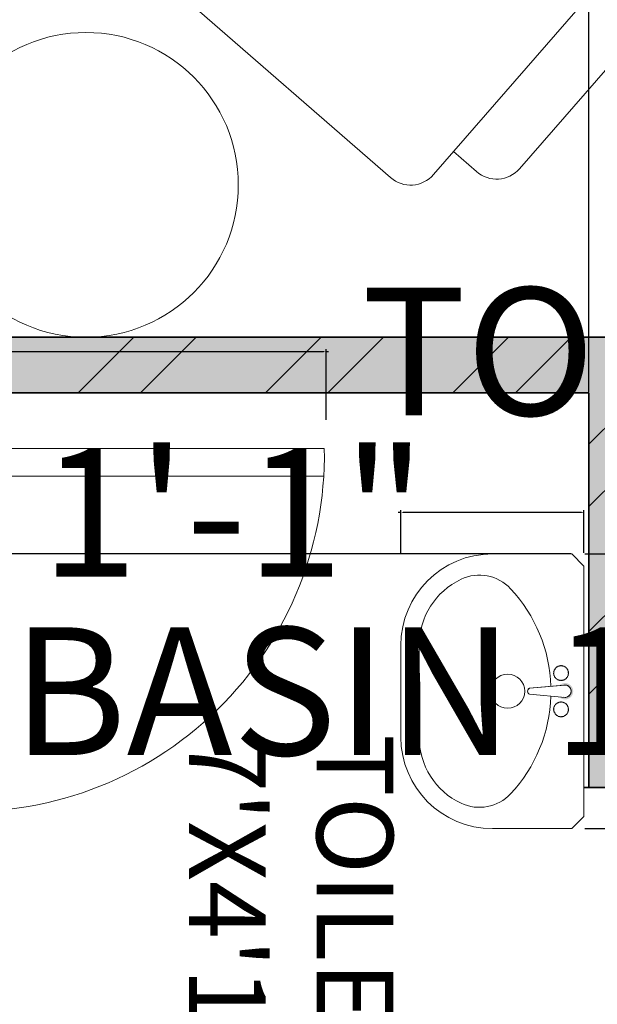
# Model space of a CAD drawing. Units: inches. Extents: x 1086 to 1540, y 3343 to 3848.
# Tile 4 of 8: x 1381 to 1422, y 3591 to 3661. Entities that reach past the tile are written whole.
import ezdxf

# ---------------------------------------------------------------- set-up
doc = ezdxf.new("R2010")
doc.units = ezdxf.units.IN
for name, color, linetype, lineweight in [('00 FURNITURE', 15, 'Continuous', 15), ('A-ANNO-DIMS', 2, 'Continuous', 13), ('A-AREA-IDEN', 7, 'Continuous', 18), ('A-DOOR', 4, 'Continuous', 20), ('A-FLOR-FIXT', 9, 'Continuous', 18), ('A-WALL-PATT', 252, 'Continuous', 9), ('A_FUR 1', 5, 'Continuous', 5), ('WALL', 7, 'Continuous', 35)]:
    doc.layers.add(name, color=color, linetype=linetype, lineweight=lineweight)
doc.styles.get("Standard").update_dxf_attribs({"font": 'arial.ttf'})
doc.dimstyles.get("Standard").update_dxf_attribs({"dimtxt": 9.18, "dimasz": 0.18, "dimexe": 0.18, "dimexo": 0.0625, "dimgap": 0.09, "dimtad": 0, "dimtih": 1, "dimtoh": 1, "dimdec": 1, "dimzin": 0, "dimdsep": 46, "dimlunit": 3, "dimtxsty": 'Standard', "dimcen": 0.09, "dimadec": 0, "dimazin": 0, "dimtfac": 1, "dimtdec": 1, "dimtofl": 0, "dimtmove": 0, "dimatfit": 3, "dimfxl": 1, "dimtolj": 1, "dimtzin": 0, "dimarcsym": 0})

# ---------------------------------------------------------------- blocks, each defined once
blk = doc.blocks.new('s_46')
at = {"ltscale": 600}
h = blk.add_hatch(color=256, dxfattribs=at)
edge = h.paths.add_edge_path()
edge.add_line((13.45184378023259, 62.04360352296498), (14.15927104179718, 54.09782096462731))
edge.add_ellipse((4.212458010588306, 52.31250418393756), major_axis=(-10.10576298371302, 2.5e-15), ratio=1, start_angle=540, end_angle=550.1754626554052, ccw=False)
edge.add_arc((4.212458010588306, 52.31250418393756), 10.10576298371302, 270, 360, ccw=False)
edge.add_line((4.212458010588306, 42.20674120020703), (4.212458010588306, 41.28018079043977))
edge.add_line((4.212458010588306, 41.28018079040339), (11.85106942148559, 41.28018079040339))
edge.add_arc((4.212458010588306, 52.31250418393756), 13.41866400745597, 664.6981342835142, 766.4847699121552)
h.paths.add_polyline_path([(4.212458010588306, 41.28018079040339), (-3.426153400272596, 41.28018079040339, 0.152566653256377), (4.212458010588306, 38.8938401764608)])
h.paths.add_polyline_path([(11.85106942144921, 41.28018079040339), (4.212458010588306, 41.28018079040339), (4.212458010588306, 38.8938401764608, 0.1525666532563772)])
h.paths.add_polyline_path([(-5.734355020395014, 54.09782096461277), (-5.026927758881356, 62.04360352296498, 0.4758332592079194), (-3.426153400272596, 41.28018079040339), (4.212458010588306, 41.28018079040339), (4.212458010588306, 42.20674120020703, -0.4672400657637396)])
for p, q in [((-5.893304973142221, 52.31250418385025), (-0.714987907151226, 110.4750654234667)), ((-5.893304973142221, 52.31250418385025), (-0.714987907151226, 110.4750654234667)), ((9.139903928502463, 110.475065423554), (14.15927104174625, 54.09782096461277)), ((14.31822099431883, 52.31250418385025), (9.139903928502463, 110.475065423554)), ((14.15927104174625, 54.09782096461277), (14.31822099431883, 52.31250418385025))]:
    blk.add_line(p, q, dxfattribs=at)
blk.add_lwpolyline([(-220.7875419894117, 171.2801807903452, -0.4142135623730951), (-70.7875419894117, 321.2801807903452), (79.2124580105883, 321.2801807904325, -0.4142135623730951), (229.2124580105883, 171.2801807904325), (229.2124580105883, 41.28018079040339), (209.2124580107047, 21.2801807904325), (-200.7875419893535, 21.28018079034518), (-220.7875419894117, 41.28018079040339)], format="xyb", close=True, dxfattribs=at)
blk.add_lwpolyline([(12.26164246437838, 75.41187665969483, 0.1816379869150311), (172.1859176590806, 141.5383421540609, 0.3263505073803008), (187.6570333366981, 222.6589125997853, 0.2898144196813102), (79.21245801076293, 291.2801807904325), (-70.78754198923707, 291.2801807903452, 0.2898144196813102), (-179.2321173155214, 222.658912599698, 0.3263505073803008), (-163.7610016377293, 141.5383421540609, 0.1816379869150315), (-3.836726442852523, 75.41187665960751)], format="xyb", dxfattribs=at)
for points in [[(-16.83803374727722, 67.43055756771354), (-17.02338931558188, 67.50428807432763), (-17.22058725368697, 67.56961317334208), (-17.42189012444578, 67.6347039079701), (-17.61956049106084, 67.70773132116301), (-17.80586091603618, 67.79686645595939), (-17.97305396257434, 67.91028035557245), (-18.11578784312587, 68.05326030802098), (-18.23825336818117, 68.21955858168076), (-18.34702699835179, 68.40004368982045), (-18.44868519355077, 68.58558414605795), (-18.54980441438965, 68.76704846357461), (-18.65696112113073, 68.9353051558137), (-18.77673177386168, 69.08122273621848), (-18.91569283319404, 69.19566971814493), (-19.07841429975815, 69.27267628890695), (-19.26144033775199, 69.31891933156292), (-19.45930865121772, 69.34423740339116), (-19.66655694507062, 69.35846906132065), (-19.87772292352747, 69.37145286262967), (-20.08734429115429, 69.39302736415993), (-20.2899587523425, 69.43303112310241), (-20.48010401183274, 69.50130269664805), (-20.65391131333308, 69.60429419830325), (-20.81388605764368, 69.73491196823306), (-20.96412718523061, 69.8826759030926), (-21.10873363655992, 70.03710589953698), (-21.25180435174844, 70.18772185422131), (-21.39743827126222, 70.3240436638007), (-21.54973433539272, 70.43559122501756), (-21.71279148443137, 70.5118844343524), (-21.88955151231494, 70.54600451889564), (-22.07832762773614, 70.54527802669325), (-22.27627589285839, 70.52059283622657), (-22.4805523698451, 70.48283682571491), (-22.68831312085968, 70.44289787355228), (-22.89671420806553, 70.41166385821998), (-23.10291169380071, 70.40002265802468), (-23.30406164005399, 70.41886215136037), (-23.49802141042892, 70.4753938675276), (-23.68545357254334, 70.56212393892929), (-23.86772199510597, 70.66788214896224), (-24.04619054717477, 70.78149828102323), (-24.22222309763311, 70.89180211850908), (-24.39718351518968, 70.98762344472925), (-24.57243566872785, 71.05779204316786), (-24.74934342730558, 71.09113769704709), (-24.92903553397628, 71.08022740500746), (-25.11170022917213, 71.03257702605333), (-25.2972906283685, 70.95943963443278), (-25.48575984616764, 70.8720683044812), (-25.67706099752104, 70.7817161102721), (-25.87114719772944, 70.69963612605352), (-26.0679715613951, 70.63708142607356), (-26.26748720381875, 70.60530508466763), (-26.46941223740578, 70.61182491958607), (-26.67252476507565, 70.64921772302478), (-26.87536788737634, 70.70632503094384), (-27.07648470485583, 70.77198837930337), (-27.27441831788747, 70.8350493038015), (-27.46771182701923, 70.88434934031102), (-27.6549083327991, 70.90873002487933), (-27.83455093560042, 70.8970328932919), (-28.00620139669627, 70.84190539614065), (-28.17349611973623, 70.75121864315588), (-28.34109016874572, 70.63664965887438), (-28.51363860827405, 70.50987546765828), (-28.69579650234664, 70.38257309404435), (-28.89221891516354, 70.26641956248204), (-29.10756091127405, 70.17309189750813), (-29.3464775547036, 70.11426712348475), (-29.61160253512208, 70.0940409177856), (-29.89748404390411, 70.0861835690448), (-30.19664889771957, 70.05688401864609), (-30.50162391323829, 69.9723312081478), (-30.80493590747938, 69.79871407902101), (-31.09911169676343, 69.50222157256212), (-31.37667809793493, 69.0490426304168), (-31.63016192783834, 68.40536619405611), (-32.32050594605971, 68.4500712644367), (-32.84873653826071, 68.3918758847285), (-33.24226493795868, 68.25193804170704), (-33.52850237919483, 68.0514157223224), (-33.73486009566113, 67.8114669136994), (-33.88874932087492, 67.5532496026135), (-34.01758128887741, 67.29792177610216), (-34.14876723336056, 67.06664142102818), (-34.30371923936764, 66.87550954936887), (-34.47985279804561, 66.72039927294827), (-34.66858425136889, 66.59212672835565), (-34.86132994201034, 66.48150805244222), (-35.04950621211901, 66.37935938188457), (-35.22452940384392, 66.27649685335928), (-35.37781585985795, 66.16373660371755), (-35.50078192248475, 66.03189476963598), (-35.58785390376579, 65.87432967920904), (-35.64549799636007, 65.69456842611542), (-35.68319036299363, 65.49868029527715), (-35.7104071660433, 65.2927345718781), (-35.73662456823513, 65.08280054092756), (-35.77131873212056, 64.87494748734753), (-35.82396582007641, 64.67524469623459), (-35.90404199482873, 64.48976145259803), (-36.01774371694773, 64.3227640100813), (-36.15814863995183, 64.17130649695173), (-36.31505471485434, 64.0306400101108), (-36.47825989319244, 63.89601564637269), (-36.63756212632871, 63.76268450255157), (-36.78275936545106, 63.62589767554891), (-36.90364956192207, 63.48090626226621), (-36.99003066710429, 63.32296135951764), (-37.03518227743916, 63.14869254492805), (-37.04631056915969, 62.96024331927765), (-37.03410336375237, 62.7611356638954), (-37.00924848217983, 62.55489156045951), (-36.98243374592858, 62.34503299021162), (-36.96434697631048, 62.13508193491725), (-36.96567599463743, 61.92856037581805), (-36.99710862222128, 61.72899029450491), (-37.06570762058254, 61.53896291530691), (-37.16403551277472, 61.35734643402975), (-37.28102976223454, 61.18207828939194), (-37.40562783187488, 61.0110959201993), (-37.52676718513249, 60.84233676508302), (-37.63338528544409, 60.67373826284892), (-37.7144195958972, 60.50323785204091), (-37.75880757992855, 60.32877297155209), (-37.75920177751686, 60.14875038337777), (-37.72311503690435, 59.96345414296957), (-37.66177528270055, 59.77363762940512), (-37.58641044021351, 59.58005422132555), (-37.5082484340528, 59.38345729780849), (-37.43851718935184, 59.18460023758234), (-37.38844463089481, 58.98423641963745), (-37.36925868364051, 58.78311922278953), (-37.38844463089481, 58.58200202594161), (-37.43851718935184, 58.38163820799673), (-37.5082484340528, 58.18278114777058), (-37.58641044021351, 57.98618422425352), (-37.66177528287517, 57.79260081626126), (-37.72311503690435, 57.6027843026095), (-37.75920177751686, 57.4174880622013), (-37.75880757992855, 57.23746547402697), (-37.7144195958972, 57.06300059353816), (-37.63338528544409, 56.89250018273014), (-37.52676718530711, 56.72390168049606), (-37.40562783187488, 56.55514252537978), (-37.28102976223454, 56.38416015618713), (-37.16403551277472, 56.20889201154932), (-37.06570762058254, 56.02727553035947), (-36.99710862222128, 55.83724815107416), (-36.96567599463743, 55.63767806976102), (-36.96434697631048, 55.43115651066182), (-36.98243374592858, 55.22120545536745), (-37.00924848217983, 55.01134688520687), (-37.03410336375237, 54.80510278168367), (-37.04631056933431, 54.60599512638873), (-37.03518227743916, 54.41754590065102), (-36.99003066710429, 54.24327708606142), (-36.90364956192207, 54.08533218331285), (-36.78275936545106, 53.94034077003016), (-36.63756212632871, 53.80355394302751), (-36.47825989319244, 53.67022279920639), (-36.31505471502896, 53.53559843546827), (-36.15814863995183, 53.39493194862734), (-36.01774371712236, 53.24347443549777), (-35.90404199482873, 53.07647699298104), (-35.82396582007641, 52.89099374934449), (-35.77131873212056, 52.69129095823155), (-35.73662456823513, 52.48343790465151), (-35.71040716621792, 52.27350387370098), (-35.68319036299363, 52.06755815021461), (-35.64549799653469, 51.87167001946363), (-35.58785390376579, 51.69190876637003), (-35.50078192248475, 51.53434367594309), (-35.3778353385278, 51.40284301002975), (-35.22468523163116, 51.29247093791491), (-35.05003213009331, 51.19609060572111), (-34.86257656256203, 51.10656515930895), (-34.67101905716118, 51.01675774488831), (-34.48406014236389, 50.91953150840708), (-34.31040034646867, 50.80774959607516), (-34.15874019777402, 50.67427515375311), (-34.03505195630714, 50.51453334218241), (-33.93439480883535, 50.3341973797942), (-33.84909967368003, 50.14150249981321), (-33.77149746881332, 49.94468393520219), (-33.69391911290586, 49.75197691909852), (-33.60869552427903, 49.57161668455228), (-33.50815762107959, 49.41183846470085), (-33.38463632145431, 49.28087749250699), (-33.23284944484476, 49.18408373402781), (-33.05706241185544, 49.11526608630083), (-32.86392754490953, 49.06534817945794), (-32.66009716555709, 49.02525364354369), (-32.45222359569743, 48.98590610860265), (-32.24695915722987, 48.93822920459206), (-32.05095617187908, 48.87314656155649), (-31.870866961719, 48.78158180962782), (-31.71133844077122, 48.65761859554914), (-31.5689958925941, 48.50798063381808), (-31.43845919286832, 48.34255165536887), (-31.31434821744915, 48.17121539139771), (-31.19128284219187, 48.00385557310073), (-31.06388294277713, 47.85035593167413), (-30.92676839523483, 47.72060019822674), (-30.77455907507101, 47.62447210386745), (-30.60346923320321, 47.56846716045401), (-30.41609062027419, 47.54552800310193), (-30.21660936163971, 47.54520904741366), (-30.00921158283018, 47.55706470907898), (-29.79808340937598, 47.570649403875), (-29.58741096680751, 47.57551754757878), (-29.38138038065517, 47.56122355579281), (-29.18417777627474, 47.51732184420689), (-28.99883273948217, 47.43692629240103), (-28.8237486963626, 47.32738863455597), (-28.65617253311211, 47.19962006882997), (-28.49335113610141, 47.06453179311938), (-28.33253139152657, 46.9330350055825), (-28.1709601857583, 46.81604090429027), (-28.00588440499268, 46.72446068713907), (-27.83455093577504, 46.66920555219985), (-27.6549083327991, 46.65750842061243), (-27.46771182701923, 46.68188910518074), (-27.27441831788747, 46.73118914177758), (-27.07648470485583, 46.7942500662757), (-26.87536788755096, 46.85991341454792), (-26.67252476525027, 46.91702072246698), (-26.4694122375804, 46.95441352590569), (-26.26748720399337, 46.96093336082412), (-26.06797156156972, 46.9291570194182), (-25.87114719772944, 46.86660231943824), (-25.67706099769566, 46.78452233530697), (-25.48575984616764, 46.69417014101054), (-25.2972906283685, 46.60679881105898), (-25.11170022934675, 46.53366141943843), (-24.92903553397628, 46.4860110404843), (-24.74934342730558, 46.47510074844467), (-24.57243566890247, 46.50844640232389), (-24.39718351536431, 46.57861500076251), (-24.22222309780773, 46.67443632698268), (-24.0461905473494, 46.78474016446853), (-23.86772199528059, 46.89835629652953), (-23.68545357254334, 47.00411450656247), (-23.49802141060354, 47.09084457796416), (-23.30406164022861, 47.14737629413138), (-23.10291169380071, 47.16621578746708), (-22.89671420806553, 47.15457458727178), (-22.68831312085968, 47.12334057193948), (-22.4805523698451, 47.08340161977685), (-22.27627589285839, 47.04564560926519), (-22.07832762791077, 47.02096041871118), (-21.88955151248956, 47.02023392650881), (-21.71279148443137, 47.05435401113937), (-21.54973433539272, 47.1306472204742), (-21.39743827126222, 47.24219478160375), (-21.25180435174844, 47.37851659118314), (-21.10873363655992, 47.52913254586746), (-20.96412718540523, 47.68356254231185), (-20.81388605764368, 47.83132647717138), (-20.65391131333308, 47.9619442471012), (-20.48010401200736, 48.0649357488437), (-20.28995875251712, 48.13320732230204), (-20.08734429115429, 48.17321108133183), (-19.87772292352747, 48.1947855828621), (-19.66655694507062, 48.2077693840838), (-19.45930865139235, 48.2220010421006), (-19.26144033775199, 48.24731911384152), (-19.07841429993277, 48.29356215667212), (-18.91569283319404, 48.37056872743414), (-18.77673177403631, 48.48501570936059), (-18.65696112113073, 48.63093328976538), (-18.54980441456428, 48.79918998200446), (-18.44868519372539, 48.98065429960843), (-18.34702699835179, 49.16619475575862), (-18.2382533683558, 49.34667986398562), (-18.11578784312587, 49.5129781376454), (-17.97305396274896, 49.6559580900066), (-17.8058609162108, 49.76937198961969), (-17.61956049106084, 49.85850712450337), (-17.4218901246204, 49.93153453769628), (-17.22058725368697, 49.996625272237), (-17.02338931558188, 50.06195037133875), (-16.83803374727722, 50.13568087795284), (-16.67225798609434, 50.22598783511785), (-16.53379946883069, 50.34104228604701), (-16.42766593385022, 50.48645191569812), (-16.34794632298872, 50.65757097714231), (-16.28599987912457, 50.84719036528259), (-16.23318584513618, 51.04810097528389), (-16.18086346407654, 51.25309370196191), (-16.12039197882404, 51.45495944039431), (-16.04313063243171, 51.64648908557137), (-15.94043866742868, 51.82047353248345), (-15.8067031877581, 51.97190354572376), (-15.64842273970134, 52.10456936812261), (-15.47512373042991, 52.22446111202589), (-15.29633256676607, 52.33756888969219), (-15.12157565605594, 52.44988281364204), (-14.96037940529641, 52.567392996134), (-14.82227022130973, 52.69608954960131), (-14.71677451161667, 52.84196258638985), (-14.6501372611965, 53.00919824198354), (-14.61547776852967, 53.19476674450561), (-14.60263391025364, 53.3938343450427), (-14.60144356318051, 53.60156729485606), (-14.60174460412236, 53.81313184503233), (-14.59337490954203, 54.02369424700736), (-14.566172356077, 54.22842075169319), (-14.50997482053935, 54.42247761052567), (-14.41809999983525, 54.6024088327249), (-14.29778487142175, 54.77026946117985), (-14.1597462335485, 54.92949229647638), (-14.01470088359201, 55.08351013963693), (-13.87336561962729, 55.23575579150929), (-13.7464572393801, 55.38966205302859), (-13.64469254092546, 55.54866172495531), (-13.5787883218145, 55.71618760822457), (-13.55583441938506, 55.89474125843844), (-13.56841282837558, 56.08309925056528), (-13.60547858278733, 56.27910691397847), (-13.65598671662155, 56.48060957840062), (-13.70889226370491, 56.68545257346704), (-13.7531502583879, 56.89148122872575), (-13.7777157346718, 57.09654087381204), (-13.77154372638324, 57.29847683827393), (-13.72730239736847, 57.49560352915432), (-13.65251243085367, 57.68811166286468), (-13.55840763938613, 57.8766610333987), (-13.45622183586238, 58.06191143448813), (-13.35718883317895, 58.24452266012667), (-13.27254244388314, 58.42515450413339), (-13.2135164810461, 58.60446676041465), (-13.19134475721512, 58.78311922278953), (-13.2135164810461, 58.96177168516442), (-13.27254244388314, 59.14108394144569), (-13.35718883317895, 59.3217157854524), (-13.45622183586238, 59.50432701109093), (-13.55840763938613, 59.68957741218037), (-13.65251243085367, 59.87812678271438), (-13.72730239736847, 60.07063491642475), (-13.77154372638324, 60.26776160730515), (-13.7777157346718, 60.46969757176703), (-13.7531502583879, 60.67475721685332), (-13.70889226370491, 60.88078587211203), (-13.65598671662155, 61.08562886717845), (-13.60547858278733, 61.2871315316006), (-13.56841282837558, 61.48313919501379), (-13.55583441938506, 61.67149718714063), (-13.5787883218145, 61.8500508373545), (-13.64469254092546, 62.01757672062377), (-13.7464572393801, 62.17657639255048), (-13.87336561962729, 62.33048265406978), (-14.01470088359201, 62.48272830594214), (-14.15974623337388, 62.63674614910269), (-14.29778487142175, 62.79596898448653), (-14.41809999983525, 62.96382961285416), (-14.50997482053935, 63.14376083514071), (-14.566172356077, 63.33781769388588), (-14.59337490936741, 63.5425441985717), (-14.60174460412236, 63.75310660054674), (-14.60144356318051, 63.96467115081032), (-14.60263391025364, 64.17240410053635), (-14.61547776835505, 64.37147170116077), (-14.65013726102188, 64.55704020359553), (-14.71677451144205, 64.7242758591892), (-14.82227022130973, 64.87014889597776), (-14.96037940529641, 64.99884544944507), (-15.12157565605594, 65.11635563193704), (-15.29633256676607, 65.22866955588688), (-15.47512373042991, 65.3417773336405), (-15.64842273970134, 65.46166907745646), (-15.8067031877581, 65.59433489985531), (-15.94043866742868, 65.74576491309563), (-16.04313063225709, 65.9197493600077), (-16.12039197882404, 66.11127900527208), (-16.18086346407654, 66.31314474370447), (-16.23318584513618, 66.5181374703825), (-16.28599987912457, 66.71904808029649), (-16.34794632298872, 66.90866746843676), (-16.42766593385022, 67.07978652988095), (-16.53379946883069, 67.22519615953206), (-16.67225798609434, 67.34025061046123)], [(22.08090273779817, 61.08562886709115), (22.03039460413856, 61.2871315315133), (21.99332884972682, 61.48313919501379), (21.9807504407363, 61.67149718705331), (22.00370434316574, 61.85005083726719), (22.06960856210208, 62.01757672053645), (22.17137326073134, 62.17657639246318), (22.29828164080391, 62.33048265398247), (22.43961690476863, 62.48272830585483), (22.58466225472512, 62.63674614901538), (22.72270089277299, 62.79596898439923), (22.84301602118649, 62.96382961276686), (22.93489084189059, 63.1437608350534), (22.99108837742824, 63.33781769379857), (23.01829093071865, 63.5425441985717), (23.0266606254736, 63.75310660045943), (23.02635958453175, 63.96467115072301), (23.02754993160488, 64.17240410053635), (23.04039378970629, 64.37147170107346), (23.07505328237312, 64.55704020350822), (23.14169053279329, 64.72427585910191), (23.24718624266097, 64.87014889589045), (23.38529542664764, 64.99884544935776), (23.54649167740717, 65.11635563193704), (23.7212485881173, 65.22866955579956), (23.90003975178115, 65.34177733355318), (24.07333876105258, 65.46166907736915), (24.23161920910934, 65.594334899768), (24.36535468877992, 65.74576491300832), (24.46804665360833, 65.9197493600077), (24.54530800017528, 66.11127900518477), (24.60577948542777, 66.31314474361714), (24.65810186648742, 66.51813747029519), (24.71091590047581, 66.71904808020918), (24.77286234433996, 66.90866746834945), (24.85258195520146, 67.07978652979364), (24.95871549018193, 67.22519615953206), (25.09717400744558, 67.34025061046123), (25.26294976862846, 67.43055756771354), (25.44830533693312, 67.50428807432763), (25.64550327503821, 67.56961317334208), (25.84680614579702, 67.6347039079701), (26.04447651241208, 67.70773132116301), (26.23077693756204, 67.79686645595939), (26.3979699841002, 67.91028035557245), (26.54070386447711, 68.05326030802098), (26.66316938970704, 68.21955858168076), (26.77194301970303, 68.40004368982045), (26.87360121507663, 68.58558414605795), (26.97472043591552, 68.76704846357461), (27.08187714248197, 68.9353051558137), (27.20164779538754, 69.08122273621848), (27.34060885454528, 69.19566971814493), (27.50333032128401, 69.27267628890695), (27.68635635910323, 69.31891933165025), (27.88422467274358, 69.34423740347847), (28.09147296642186, 69.35846906140794), (28.30263894487871, 69.37145286262967), (28.51226031250553, 69.39302736424725), (28.71487477386836, 69.43303112318972), (28.90502003318398, 69.50130269673537), (29.07882733468432, 69.60429419839056), (29.23880207899492, 69.73491196832038), (29.38904320658185, 69.88267590317992), (29.53364965791116, 70.0371058996243), (29.67672037309967, 70.18772185430862), (29.82235429261346, 70.324043663888), (29.97465035674395, 70.43559122501756), (30.1377075057826, 70.51188443443971), (30.31446753366618, 70.54600451898295), (30.50324364908738, 70.54527802678058), (30.70119191420963, 70.52059283622657), (30.90546839119634, 70.48283682571491), (31.11322914221091, 70.4428978736396), (31.32163022941677, 70.41166385830729), (31.52782771515195, 70.400022658112), (31.72897766157985, 70.41886215144768), (31.92293743178016, 70.4753938675276), (32.11036959389458, 70.56212393892929), (32.29263801663183, 70.66788214896224), (32.47110656870063, 70.78149828102323), (32.64713911898434, 70.89180211850908), (32.82209953654092, 70.98762344481656), (32.99735169025371, 71.05779204316786), (33.17425944865681, 71.09113769704709), (33.35395155532751, 71.08022740500746), (33.53661625069799, 71.03257702605333), (33.72220664971974, 70.9594396345201), (33.91067586751888, 70.8720683044812), (34.1019770190469, 70.7817161102721), (34.29606321908068, 70.69963612605352), (34.49288758292096, 70.63708142616088), (34.69240322534461, 70.60530508466763), (34.89432825893164, 70.61182491958607), (35.09744078660151, 70.64921772302478), (35.3002839089022, 70.70632503103116), (35.50140072620707, 70.77198837930337), (35.6993343392387, 70.8350493038015), (35.89262784837047, 70.88434934039833), (36.07982435415034, 70.90873002487933), (36.25946695695166, 70.8970328932919), (36.43111741804751, 70.84190539614065), (36.59841214108747, 70.75121864315588), (36.76600619009696, 70.63664965887438), (36.93855462962529, 70.50987546765828), (37.12071252369788, 70.38257309404435), (37.3171349366894, 70.26641956248204), (37.53247693262529, 70.17309189750813), (37.77139357605483, 70.11426712348475), (38.03651855647331, 70.0940409177856), (38.32240006525535, 70.0861835690448), (38.62156491907081, 70.05688401864609), (38.92653993476415, 69.9723312081478), (39.22985192883061, 69.79871407893368), (39.52402771811467, 69.50222157256212), (39.80159411928616, 69.0490426304168), (40.05507794918957, 68.4053661939688), (40.74542196741094, 68.4500712644367), (41.27365255961194, 68.3918758846412), (41.66718095948453, 68.25193804161972), (41.95341840054607, 68.0514157223224), (42.15977611701236, 67.8114669136121), (42.31366534240078, 67.5532496025262), (42.44249731022864, 67.29792177601485), (42.57368325471179, 67.06664142094087), (42.72863526071887, 66.87550954936887), (42.90476881939684, 66.72039927286096), (43.09350027272012, 66.59212672826834), (43.28624596336157, 66.48150805235491), (43.47442223347025, 66.37935938179726), (43.64944542536977, 66.27649685335928), (43.80273188138381, 66.16373660371755), (43.92569794383598, 66.03189476963598), (44.01276992511703, 65.87432967912173), (44.0704140177113, 65.69456842602813), (44.10810638434486, 65.49868029527715), (44.13532318739453, 65.2927345718781), (44.16154058958636, 65.08280054084025), (44.19623475347179, 64.87494748726021), (44.24888184142765, 64.67524469614727), (44.32895801617997, 64.48976145251072), (44.44265973829897, 64.32276400999397), (44.58306466130307, 64.17130649695173), (44.73997073620558, 64.03064001002348), (44.90317591454368, 63.89601564628538), (45.06247814767994, 63.76268450246425), (45.20767538680229, 63.6258976754616), (45.3285655832733, 63.4809062621789), (45.41494668845553, 63.32296135943034), (45.46009829879039, 63.14869254484074), (45.47122659051092, 62.96024331919034), (45.45901938492898, 62.76113566380809), (45.43416450353106, 62.5548915603722), (45.40734976727981, 62.34503299021162), (45.38926299766171, 62.13508193482994), (45.39059201598866, 61.92856037573074), (45.42202464357251, 61.7289902944176), (45.49062364193377, 61.53896291521959), (45.58895153412595, 61.35734643394243), (45.70594578341115, 61.18207828939194), (45.83054385322611, 61.01109592011198), (45.95168320648371, 60.84233676508302), (46.05830130679533, 60.67373826276162), (46.13933561724843, 60.50323785204091), (46.18372360127978, 60.32877297146479), (46.1841177988681, 60.14875038329046), (46.14803105825558, 59.96345414296957), (46.08669130405178, 59.77363762931782), (46.01132646156474, 59.58005422123824), (45.93316445540404, 59.38345729772118), (45.86343321070308, 59.18460023749503), (45.81336065224604, 58.98423641955014), (45.79417470499175, 58.78311922270222), (45.81336065224604, 58.58200202585431), (45.86343321070308, 58.38163820790942), (45.93316445540404, 58.18278114777058), (46.01132646156474, 57.98618422416621), (46.08669130405178, 57.79260081617394), (46.14803105808095, 57.6027843025222), (46.1841177988681, 57.4174880622013), (46.18372360127978, 57.23746547393966), (46.13933561724843, 57.06300059345085), (46.05830130679533, 56.89250018273014), (45.95168320648371, 56.72390168040874), (45.83054385322611, 56.55514252529247), (45.70594578341115, 56.38416015609982), (45.58895153412595, 56.20889201154932), (45.49062364193377, 56.02727553027216), (45.42202464339789, 55.83724815107416), (45.39059201598866, 55.63767806976102), (45.38926299766171, 55.43115651066182), (45.40734976727981, 55.22120545528014), (45.43416450335644, 55.01134688511957), (45.45901938492898, 54.80510278159636), (45.47122659051092, 54.60599512630142), (45.46009829879039, 54.41754590056371), (45.41494668845553, 54.24327708597411), (45.32856558309868, 54.08533218322554), (45.20767538662767, 53.94034076994285), (45.06247814750532, 53.8035539429402), (44.90317591454368, 53.67022279920639), (44.73997073620558, 53.53559843538096), (44.58306466130307, 53.39493194854004), (44.44265973829897, 53.24347443541046), (44.32895801617997, 53.07647699298104), (44.24888184125302, 52.89099374934449), (44.19623475329717, 52.69129095823155), (44.16154058958636, 52.48343790465151), (44.13532318739453, 52.27350387361366), (44.10810638434486, 52.06755815021461), (44.0704140177113, 51.87167001946363), (44.01276992511703, 51.69190876628272), (43.92569794366136, 51.53434367585578), (43.80275135970442, 51.40284301002975), (43.64960125280776, 51.29247093791491), (43.47494815144455, 51.1960906056338), (43.28749258373863, 51.10656515922165), (43.09593507851241, 51.01675774480099), (42.90897616371512, 50.91953150840708), (42.73531636764528, 50.80774959598784), (42.58365621895063, 50.67427515375311), (42.45996797765838, 50.51453334218241), (42.35931083018658, 50.3341973797942), (42.27401569485664, 50.14150249981321), (42.19641349016455, 49.94468393520219), (42.1188351342571, 49.75197691909852), (42.03361154545564, 49.57161668455228), (41.9330736422562, 49.41183846461354), (41.80955234280554, 49.28087749250699), (41.65776546602137, 49.1840837339405), (41.48197843320668, 49.11526608630083), (41.28884356608614, 49.06534817945794), (41.0850131867337, 49.02525364354369), (40.87713961687405, 48.98590610851534), (40.67187517840648, 48.93822920459206), (40.47587219323031, 48.87314656155649), (40.29578298289561, 48.78158180962782), (40.13625446194782, 48.65761859554914), (39.99391191377072, 48.50798063373076), (39.86337521404493, 48.34255165528157), (39.73926423862577, 48.17121539139771), (39.61619886336848, 48.00385557310073), (39.48879896395374, 47.85035593167413), (39.35168441641144, 47.72060019813944), (39.19947509624762, 47.62447210378013), (39.02838525455445, 47.56846716045401), (38.8410066414508, 47.54552800310193), (38.64152538281633, 47.54520904732635), (38.43412760400679, 47.55706470907898), (38.22299943072721, 47.570649403875), (38.01232698798413, 47.57551754757878), (37.80629640183179, 47.56122355579281), (37.60909379745135, 47.51732184420689), (37.42374876065878, 47.43692629240103), (37.24866471753922, 47.32738863455597), (37.08108855428873, 47.19962006882997), (36.91826715727803, 47.06453179311938), (36.75744741270319, 46.9330350056698), (36.59587620693492, 46.81604090429027), (36.4308004261693, 46.72446068713907), (36.25946695695166, 46.66920555228716), (36.07982435397571, 46.65750842061243), (35.89262784837047, 46.68188910518074), (35.6993343392387, 46.73118914177758), (35.50140072620707, 46.7942500662757), (35.30028390872758, 46.85991341454792), (35.09744078642689, 46.91702072246698), (34.89432825875701, 46.954413525993), (34.69240322516998, 46.96093336082412), (34.49288758274633, 46.9291570194182), (34.29606321908068, 46.86660231943824), (34.10197701887228, 46.78452233530697), (33.91067586734425, 46.69417014109785), (33.72220664971974, 46.60679881105898), (33.53661625052337, 46.53366141943843), (33.35395155515289, 46.4860110404843), (33.17425944865681, 46.47510074844467), (32.99735169007909, 46.5084464024112), (32.82209953654092, 46.57861500076251), (32.64713911898434, 46.67443632707), (32.47110656852601, 46.78474016446853), (32.2926380164572, 46.89835629661684), (32.11036959389458, 47.00411450664979), (31.92293743178016, 47.09084457805147), (31.72897766140522, 47.14737629413138), (31.52782771497732, 47.16621578746708), (31.32163022941677, 47.15457458727178), (31.11322914203629, 47.12334057193948), (30.90546839102171, 47.08340161986416), (30.70119191420963, 47.0456456093525), (30.50324364908738, 47.02096041879849), (30.31446753366618, 47.02023392659611), (30.1377075057826, 47.05435401113937), (29.97465035674395, 47.13064722056151), (29.82235429261346, 47.24219478169106), (29.67672037309967, 47.37851659127045), (29.53364965791116, 47.52913254595478), (29.38904320658185, 47.68356254239916), (29.2388020788203, 47.8313264772587), (29.0788273345097, 47.96194424718851), (28.90502003318398, 48.06493574893102), (28.71487477369374, 48.13320732238935), (28.51226031250553, 48.17321108133183), (28.30263894487871, 48.19478558294941), (28.09147296642186, 48.20776938417111), (27.88422467256896, 48.22200104218791), (27.68635635892861, 48.24731911392882), (27.50333032110939, 48.29356215667212), (27.34060885454528, 48.37056872743414), (27.20164779521292, 48.48501570936059), (27.08187714248197, 48.63093328976538), (26.97472043574089, 48.79918998200446), (26.87360121490201, 48.98065429960843), (26.77194301952841, 49.16619475575862), (26.66316938953241, 49.34667986398562), (26.54070386447711, 49.51297813755809), (26.39796998392558, 49.6559580900066), (26.23077693738742, 49.76937198961969), (26.04447651223745, 49.85850712450337), (25.84680614579702, 49.93153453769628), (25.64550327486359, 49.996625272237), (25.44830533675849, 50.06195037133875), (25.26294976862846, 50.13568087795284), (25.09717400727095, 50.22598783520516), (24.95871549018193, 50.34104228604701), (24.85258195520146, 50.48645191561082), (24.77286234416534, 50.657570977055), (24.71091590030119, 50.84719036519527), (24.65810186648742, 51.04810097519657), (24.60577948542777, 51.2530937018746), (24.54530800017528, 51.45495944030699), (24.46804665360833, 51.64648908548406), (24.36535468877992, 51.82047353239614), (24.23161920910934, 51.97190354572376), (24.07333876105258, 52.1045693680353), (23.90003975160653, 52.22446111193858), (23.7212485881173, 52.33756888960488), (23.54649167740717, 52.44988281355472), (23.38529542647302, 52.56739299604669), (23.24718624266097, 52.696089549514), (23.14169053279329, 52.84196258630254), (23.07505328237312, 53.00919824189623), (23.04039378970629, 53.1947667444183), (23.02754993160488, 53.39383434495539), (23.02635958453175, 53.60156729476876), (23.02666062529898, 53.81313184503233), (23.01829093071865, 54.02369424692006), (22.99108837725362, 54.22842075169319), (22.93489084171597, 54.42247761043836), (22.84301602101186, 54.6024088327249), (22.72270089277299, 54.77026946109254), (22.58466225472512, 54.92949229638907), (22.43961690476863, 55.08351013963693), (22.29828164080391, 55.23575579150929), (22.17137326073134, 55.38966205294127), (22.06960856210208, 55.548661724868), (22.00370434316574, 55.71618760813726), (21.9807504407363, 55.89474125843844), (21.99332884972682, 56.08309925047797), (22.03039460413856, 56.27910691389115), (22.08090273779817, 56.48060957840062), (22.13380828505615, 56.68545257346704), (22.17806627973914, 56.89148122872575), (22.20263175602304, 57.09654087381204), (22.19645974773448, 57.29847683827393), (22.15221841871971, 57.49560352915432), (22.07742845220491, 57.68811166286468), (21.98332366073737, 57.87666103331139), (21.88113785721362, 58.06191143448813), (21.78210485453019, 58.24452266012667), (21.69745846523438, 58.42515450413339), (21.63843250239734, 58.60446676032734), (21.61626077856636, 58.78311922270222), (21.63843250239734, 58.96177168507711), (21.69745846523438, 59.14108394135837), (21.78210485453019, 59.32171578536508), (21.88113785721362, 59.50432701100362), (21.98332366073737, 59.68957741209306), (22.07742845220491, 59.87812678262708), (22.15221841871971, 60.07063491633743), (22.19645974773448, 60.26776160721784), (22.20263175602304, 60.46969757167971), (22.17806627973914, 60.67475721676601), (22.13380828505615, 60.88078587202471)]]:
    blk.add_lwpolyline(points, close=True, dxfattribs=at)
blk.add_circle((4.212458010588306, 146.2801807904034), 28, dxfattribs=at)
for centre, radius, start, end in [((4.212458010588306, 108.2109541267855), 5.422722861947412, 24.67830004152974, 155.3216999584702), ((4.212458010588306, 52.31250418393756), 10.10576298371233, 169.8245373479931, 0)]:
    blk.add_arc(centre, radius, start, end, dxfattribs=at)
for centre, major_axis, ratio, start_param, end_param in [((4.212458010762929, 110.475065423554), (-4.927445917859709, 1.2e-15), 0.6410240960233505, 3.141592653589793, 6.283185307179586), ((4.212458010588306, 52.31250418393756), (-10.10576298371302, 2.5e-15), 1, 6.105589980929039, 9.602373287019926)]:
    blk.add_ellipse(centre, major_axis=major_axis, ratio=ratio, start_param=start_param, end_param=end_param, dxfattribs=at)
blk = doc.blocks.new('ESTSET')
at = {"layer": 'A_FUR 1'}
for p, q in [((-10.44359699611232, 4.096573562603225), (-10.44359699611232, 32.09657356260323)), ((-8.44359699611232, 4.096573562603225), (-8.44359699611232, 32.09657356260323)), ((-36.44359699611232, 6.096573562603225), (-36.44359699611232, 3.096573562603225)), ((-34.44359699611232, 6.096573562603225), (-36.44359699611232, 6.096573562603225)), ((-34.44359699611232, 4.096573562603225), (-34.44359699611232, 6.096573562603225)), ((-34.44359699611232, 4.096573562603225), (-34.44359699611232, 6.096573562603225)), ((-8.44359699611232, 4.096573562603225), (-8.44359699611232, 6.096573562603225)), ((-8.44359699611232, 6.096573562603225), (-6.443596996112319, 6.096573562603225)), ((-8.44359699611232, 4.096573562603225), (-8.44359699611232, 6.096573562603225)), ((-6.443596996112319, 6.096573562603225), (-6.443596996112319, 3.096573562603225)), ((-32.44359699611232, 4.096573562603225), (-34.44359699611232, 4.096573562603225)), ((-32.44359699611232, 4.096573562603225), (-34.44359699611232, 4.096573562603225)), ((-32.44359699611232, 3.096573562603225), (-32.44359699611232, 4.096573562603225)), ((-10.44359699611232, 3.096573562603225), (-10.44359699611232, 4.096573562603225)), ((-10.44359699611232, 4.096573562603225), (-8.44359699611232, 4.096573562603225)), ((-10.44359699611232, 4.096573562603225), (-8.44359699611232, 4.096573562603225)), ((-6.443596996112319, 2.096573562601521), (-36.4435969961196, 2.09657356260334)), ((-35.44359699611232, 2.096573562603225), (-33.44359699611232, 2.096573562603225)), ((-7.443596996112319, 2.096573562603225), (-9.44359699611232, 2.096573562603225))]:
    blk.add_line(p, q, dxfattribs=at)
for points in [[(-21.44359699614506, 2.09657356260334), (-18.67227073841423, 2.09657356260334), (-18.67227073841423, 5.101808480258228), (-20.05793386727964, 5.101808480258228)], [(-20.05793386727964, 5.101808480258228), (-20.05793386727964, -0.9086613550515485)], [(-21.44359699614506, 2.09657356260334), (-21.44359699614506, -0.9086613550515485), (-20.05793386727964, -0.9086613550515485)]]:
    blk.add_lwpolyline(points, dxfattribs=at)
for centre, radius, start, end in [((-8.908777800232201, 6.457098594999479), 25.64369454261379, 88.96058819788949, 185.2816045955121), ((-35.44359699611232, 3.096573562603225), 1, 180, 270), ((-33.44359699611232, 3.096573562603225), 1, 270, 0), ((-9.44359699611232, 3.096573562603225), 1, 180, 270), ((-7.443596996112319, 3.096573562603225), 1, 270, 0)]:
    blk.add_arc(centre, radius, start, end, dxfattribs=at)
blk = doc.blocks.new('chair')
at = {"layer": '00 FURNITURE'}
for p, q in [((1375.845081742341, 3529.745138182322), (1402.123430747959, 3529.745138182322)), ((1373.655238967809, 3525.365452633256), (1373.655238967809, 3527.555295407789)), ((1371.465396193043, 3525.365452633256), (1397.743745198893, 3525.365452633256)), ((1369.275553418511, 3501.277182112698), (1369.275553418511, 3523.175609858724))]:
    blk.add_line(p, q, dxfattribs=at)
for centre in [(1375.845081742341, 3527.555295407789), (1371.465396193043, 3523.175609858724)]:
    blk.add_arc(centre, 2.189842774590119, 90, 180, dxfattribs=at)
blk = doc.blocks.new('TABLE-ROUND-SIDE')
blk.add_circle((2.274e-13, 0), 10.94980314960581)
blk = doc.blocks.new('*D32')
at = {"layer": 'A-ANNO-DIMS', "color": 0, "lineweight": -2, "transparency": 16777216}
for p, q in [((1437.74044790643, 3674.099188760906), (1437.74044790643, 3668.063883562158)), ((1461.74044790643, 3674.099188760906), (1461.74044790643, 3668.063883562158)), ((1437.74044790643, 3668.243883562158), (1437.56044790643, 3668.243883562158)), ((1461.56044790643, 3668.243883562158), (1437.92044790643, 3668.243883562158))]:
    blk.add_line(p, q, dxfattribs=at)
at = {"layer": 'A-ANNO-DIMS', "color": 0, "transparency": 16777216}
for points in [[(1437.92044790643, 3668.273883562159), (1437.92044790643, 3668.213883562158), (1437.74044790643, 3668.243883562158)], [(1461.56044790643, 3668.273883562159), (1461.56044790643, 3668.213883562158), (1461.74044790643, 3668.243883562158)]]:
    blk.add_solid(points, dxfattribs=at)
at = {"layer": 'Defpoints', "color": 0, "transparency": 16777216}
for p in [(1437.74044790643, 3674.161688760906), (1461.74044790643, 3674.161688760906), (1437.74044790643, 3668.243883562158)]:
    blk.add_point(p, dxfattribs=at)
at = {"layer": 'A-ANNO-DIMS', "color": 0, "transparency": 16777216, "insert": (1409.413838083783, 3668.243883562158), "char_height": 9.18, "attachment_point": 5}
blk.add_mtext('\\A1;2\'-0" TYP.', dxfattribs=at)
blk = doc.blocks.new('*D37')
at = {"layer": 'A-ANNO-DIMS', "color": 0, "lineweight": -2, "transparency": 16777216}
for p, q in [((1421.441194156199, 3622.996804096682), (1424.520541861364, 3622.996804096682)), ((1424.340541861364, 3622.816804096682), (1424.340541861364, 3617.960526843904)), ((1424.340541861364, 3603.431152728914), (1424.340541861364, 3608.287429981693)), ((1421.441194156199, 3603.251152728914), (1424.520541861364, 3603.251152728914))]:
    blk.add_line(p, q, dxfattribs=at)
at = {"layer": 'A-ANNO-DIMS', "color": 0, "transparency": 16777216}
for points in [[(1424.310541861364, 3622.816804096682), (1424.370541861364, 3622.816804096682), (1424.340541861364, 3622.996804096682)], [(1424.310541861364, 3603.431152728914), (1424.370541861364, 3603.431152728914), (1424.340541861364, 3603.251152728914)]]:
    blk.add_solid(points, dxfattribs=at)
at = {"layer": 'Defpoints', "color": 0, "transparency": 16777216}
for p in [(1421.378694156199, 3622.996804096682), (1424.340541861364, 3622.996804096682), (1421.378694156199, 3603.251152728914)]:
    blk.add_point(p, dxfattribs=at)
at = {"layer": 'A-ANNO-DIMS', "color": 0, "transparency": 16777216, "insert": (1424.340541861365, 3613.123978412796), "char_height": 9.18, "attachment_point": 5}
blk.add_mtext('\\A1;BASIN 1\'-7 1/2"', dxfattribs=at)
blk = doc.blocks.new('*D38')
at = {"layer": 'A-ANNO-DIMS', "color": 0, "lineweight": -2, "transparency": 16777216}
for p, q in [((1408.214926577682, 3625.958651801846), (1408.034926577682, 3625.958651801846)), ((1408.214926577682, 3623.05930409668), (1408.214926577682, 3626.138651801845)), ((1421.198694156198, 3625.958651801846), (1408.394926577682, 3625.958651801846)), ((1421.378694156198, 3623.05930409668), (1421.378694156198, 3626.138651801845))]:
    blk.add_line(p, q, dxfattribs=at)
at = {"layer": 'A-ANNO-DIMS', "color": 0, "transparency": 16777216}
for points in [[(1408.394926577682, 3625.988651801846), (1408.394926577682, 3625.928651801846), (1408.214926577682, 3625.958651801846)], [(1421.198694156198, 3625.988651801846), (1421.198694156198, 3625.928651801846), (1421.378694156198, 3625.958651801846)]]:
    blk.add_solid(points, dxfattribs=at)
at = {"layer": 'Defpoints', "color": 0, "transparency": 16777216}
for p in [(1408.214926577682, 3625.958651801846), (1408.214926577682, 3622.99680409668), (1421.378694156198, 3622.99680409668)]:
    blk.add_point(p, dxfattribs=at)
at = {"layer": 'A-ANNO-DIMS', "color": 0, "transparency": 16777216, "insert": (1396.175615527205, 3625.958651801846), "char_height": 9.18, "attachment_point": 5}
blk.add_mtext('\\A1;1\'-1"', dxfattribs=at)
blk = doc.blocks.new('*D41')
at = {"layer": 'A-ANNO-DIMS', "color": 0, "lineweight": -2, "transparency": 16777216}
for p, q in [((1369.709395983253, 3632.633280204329), (1369.709395983253, 3637.721409000223)), ((1402.846921289218, 3632.633280204329), (1402.846921289218, 3637.721409000223)), ((1369.889395983253, 3637.541409000223), (1402.666921289218, 3637.541409000223)), ((1402.846921289218, 3637.541409000223), (1403.026921289218, 3637.541409000223))]:
    blk.add_line(p, q, dxfattribs=at)
at = {"layer": 'A-ANNO-DIMS', "color": 0, "transparency": 16777216}
for points in [[(1369.889395983253, 3637.571409000223), (1369.889395983253, 3637.511409000223), (1369.709395983253, 3637.541409000223)], [(1402.666921289218, 3637.571409000223), (1402.666921289218, 3637.511409000223), (1402.846921289218, 3637.541409000223)]]:
    blk.add_solid(points, dxfattribs=at)
at = {"layer": 'Defpoints', "color": 0, "transparency": 16777216}
for p in [(1402.846921289218, 3637.541409000223), (1369.709395983253, 3632.570780204329), (1402.846921289218, 3632.570780204329)]:
    blk.add_point(p, dxfattribs=at)
at = {"layer": 'A-ANNO-DIMS', "color": 0, "transparency": 16777216, "insert": (1460.679779406544, 3637.541409000223), "char_height": 9.18, "attachment_point": 5}
blk.add_mtext('\\A1;TOILET DOOR 2\'-9"', dxfattribs=at)
blk = doc.blocks.new('*D69')
at = {"layer": 'A-ANNO-DIMS', "color": 0, "lineweight": -2, "transparency": 16777216}
for p, q in [((1421.677948, 3634.570780000002), (1171.560448000001, 3634.570780000002)), ((1171.740448000001, 3634.390780000002), (1171.740448000001, 3633.620340431107)), ((1171.740448000001, 3623.176804000002), (1171.740448000001, 3623.947243568897)), ((1420.43861, 3622.996804000002), (1171.560448000001, 3622.996804000002))]:
    blk.add_line(p, q, dxfattribs=at)
at = {"layer": 'A-ANNO-DIMS', "color": 0, "transparency": 16777216}
for points in [[(1171.710448000001, 3634.390780000002), (1171.770448000001, 3634.390780000002), (1171.740448000001, 3634.570780000002)], [(1171.710448000001, 3623.176804000002), (1171.770448000001, 3623.176804000002), (1171.740448000001, 3622.996804000002)]]:
    blk.add_solid(points, dxfattribs=at)
at = {"layer": 'Defpoints', "color": 0, "transparency": 16777216}
for p in [(1421.740448, 3634.570780000002), (1171.740448000001, 3622.996804000002), (1420.50111, 3622.996804000002)]:
    blk.add_point(p, dxfattribs=at)
at = {"layer": 'A-ANNO-DIMS', "color": 0, "transparency": 16777216, "insert": (1171.740448000002, 3628.783792), "char_height": 9.18, "attachment_point": 5}
blk.add_mtext('\\A1;0\'-11 1/2"', dxfattribs=at)
blk = doc.blocks.new('*D70')
at = {"layer": 'A-ANNO-DIMS', "color": 0, "lineweight": -2, "transparency": 16777216}
for p, q in [((1376.740448, 3634.63328), (1376.740448, 3834.75078)), ((1376.920448, 3834.57078), (1386.952194248294, 3834.57078)), ((1421.560448, 3834.57078), (1411.528701751705, 3834.57078)), ((1421.740448, 3634.63328), (1421.740448, 3834.75078))]:
    blk.add_line(p, q, dxfattribs=at)
at = {"layer": 'A-ANNO-DIMS', "color": 0, "transparency": 16777216}
for points in [[(1376.920448, 3834.60078), (1376.920448, 3834.54078), (1376.740448, 3834.57078)], [(1421.560448, 3834.60078), (1421.560448, 3834.54078), (1421.740448, 3834.57078)]]:
    blk.add_solid(points, dxfattribs=at)
at = {"layer": 'Defpoints', "color": 0, "transparency": 16777216}
for p in [(1421.740448, 3834.57078), (1376.740448, 3634.57078), (1421.740448, 3634.57078)]:
    blk.add_point(p, dxfattribs=at)
at = {"layer": 'A-ANNO-DIMS', "color": 0, "transparency": 16777216, "insert": (1399.240448, 3834.57078), "char_height": 9.18, "attachment_point": 5}
blk.add_mtext('\\A1;3\'-9"', dxfattribs=at)

msp = doc.modelspace()

# ---------------------------------------------------------------- hatches: boundary and pattern name
at = {"layer": 'A-WALL-PATT'}
h = msp.add_hatch(dxfattribs=at)
h.set_pattern_fill('ANSI32', color=256)
h.set_pattern_definition([(45, (0, 0), (-6.735192090801865, 6.735192090801866), []), (45, (4.49013, 0), (-6.735192090801865, 6.735192090801866), [])])
h.paths.add_polyline_path([(1234.550507268797, 3811.570780184086), (1234.550506085547, 3811.570780184086), (1194.74044790643, 3811.570780204329), (1194.74044790643, 3622.570780204329), (1203.74044790643, 3622.570780204329), (1203.74044790643, 3634.57078020433), (1218.334481095046, 3634.57078020433), (1218.334481095046, 3638.570780204329), (1203.74044790643, 3638.570780204329), (1203.74044790643, 3802.570780204329), (1234.550507268797, 3802.570780204328)])
h.paths.add_polyline_path([(1371.059017457095, 3811.570780184086), (1371.059016273845, 3811.570780184086), (1282.550507268797, 3811.570780204329), (1282.550507268797, 3802.570780204328), (1331.74044790643, 3802.570780204329), (1331.74044790643, 3634.57078020433), (1335.740443663098, 3634.570780204329), (1335.740443663098, 3639.570779622127), (1335.74044790643, 3802.570780204329), (1371.059017457095, 3802.570780204329)])
h.paths.add_polyline_path([(1470.74044790643, 3811.570780204329), (1419.059017457095, 3811.570780204329), (1419.059017457094, 3802.570780204329), (1461.74044790643, 3802.570780204329), (1461.74044790643, 3638.570780204329), (1461.74044790643, 3548.570780204335), (1425.74044790643, 3548.570780204334), (1425.74044790643, 3582.213777424251), (1421.74044790643, 3582.213777424251), (1421.74044790643, 3548.570780204334), (1376.74044790643, 3548.570780204333), (1376.74044790643, 3602.570780204329), (1373.714630900908, 3602.570780204329), (1372.74044790643, 3602.570780204329), (1372.74044790643, 3544.570780204329), (1461.74044790643, 3544.570780204332), (1461.74044790643, 3379.57078020433), (1470.74044790643, 3379.570780204329)])
h.paths.add_polyline_path([(1203.74044790643, 3582.570780204329), (1295.74044790643, 3582.57078020433), (1295.74044790643, 3586.57078020433), (1203.74044790643, 3586.570780204329), (1203.74044790643, 3598.570780204329), (1194.74044790643, 3598.570780204329), (1194.74044790643, 3379.570780204329), (1326.74044790643, 3379.570780204329), (1326.74044790643, 3388.570780204329), (1322.74044790643, 3388.570780204329), (1203.74044790643, 3388.570780204329), (1203.74044790643, 3451.570780204329), (1234.74044790643, 3451.570780204329), (1234.740447906429, 3455.570780204329), (1203.74044790643, 3455.570780204329), (1203.74044790643, 3479.570780204329), (1203.74044790643, 3544.570780204329), (1227.74044790643, 3544.570780204329), (1253.74044790643, 3544.570780204329), (1253.74044790643, 3548.570780204329), (1203.74044790643, 3548.570780204329)])
h.paths.add_polyline_path([(1461.74044790643, 3638.570780204329), (1371.74044790643, 3638.570780204329), (1371.74044790643, 3634.570780204329), (1372.74044790643, 3634.57078020433), (1372.74044790643, 3632.570780204328), (1376.74044790643, 3632.570780204328), (1376.74044790643, 3634.570780204329), (1421.74044790643, 3634.57078020433), (1421.74044790643, 3606.21377742425), (1425.74044790643, 3606.213777424251), (1425.74044790643, 3634.57078020433), (1461.74044790643, 3634.57078020433)])
h.paths.add_polyline_path([(1295.740445944246, 3638.570780204329), (1266.334481095045, 3638.570780204329), (1266.334481095045, 3634.57078020433), (1292.74044790643, 3634.57078020433), (1295.740445944246, 3634.57078020433)])
h.paths.add_polyline_path([(1322.74044790643, 3548.570780204332), (1318.74044790643, 3548.570780204331), (1318.74044790643, 3455.570780204329), (1282.74044790643, 3455.570780204329), (1282.74044790643, 3451.57078020433), (1318.74044790643, 3451.57078020433), (1318.74044790643, 3420.07078020433), (1322.74044790643, 3420.07078020433)], flags=17)
at = {"layer": 'A-WALL-PATT', "transparency": 33554559}
h = msp.add_hatch(color=256, dxfattribs=at)
h.dxf.hatch_style = 1
h.paths.add_polyline_path([(1234.550507268797, 3811.570780184086), (1234.550506085547, 3811.570780184086), (1194.74044790643, 3811.570780204329), (1194.74044790643, 3622.570780204329), (1203.74044790643, 3622.570780204329), (1203.74044790643, 3634.57078020433), (1218.334481095046, 3634.57078020433), (1218.334481095046, 3638.570780204329), (1203.74044790643, 3638.570780204329), (1203.74044790643, 3802.570780204329), (1234.550507268797, 3802.570780204328)])
h.paths.add_polyline_path([(1371.059017457095, 3811.570780184086), (1371.059016273845, 3811.570780184086), (1282.550507268797, 3811.570780204329), (1282.550507268797, 3802.570780204328), (1331.74044790643, 3802.570780204329), (1331.74044790643, 3634.57078020433), (1335.740443663098, 3634.570780204329), (1335.740443663098, 3639.570779622127), (1335.74044790643, 3802.570780204329), (1371.059017457095, 3802.570780204329)])
h.paths.add_polyline_path([(1470.74044790643, 3811.570780204329), (1419.059017457095, 3811.570780204329), (1419.059017457094, 3802.570780204329), (1461.74044790643, 3802.570780204329), (1461.74044790643, 3638.570780204329), (1461.74044790643, 3548.570780204335), (1425.74044790643, 3548.570780204334), (1425.74044790643, 3582.213777424251), (1421.74044790643, 3582.213777424251), (1421.74044790643, 3548.570780204334), (1376.74044790643, 3548.570780204333), (1376.74044790643, 3602.570780204328), (1372.74044790643, 3602.570780204329), (1372.74044790643, 3544.570780204329), (1461.74044790643, 3544.570780204332), (1461.74044790643, 3379.57078020433), (1470.74044790643, 3379.570780204329)])
h.paths.add_polyline_path([(1203.74044790643, 3544.570780204329), (1227.74044790643, 3544.570780204329), (1253.74044790643, 3544.570780204329), (1253.74044790643, 3548.570780204329), (1203.74044790643, 3548.570780204329), (1203.74044790643, 3582.570780204329), (1295.74044790643, 3582.57078020433), (1295.74044790643, 3586.57078020433), (1203.74044790643, 3586.570780204329), (1203.74044790643, 3598.570780204329), (1194.74044790643, 3598.570780204329), (1194.74044790643, 3379.570780204329), (1326.74044790643, 3379.570780204329), (1326.74044790643, 3388.570780204329), (1322.74044790643, 3388.570780204329), (1203.74044790643, 3388.570780204329), (1203.74044790643, 3451.570780204329), (1234.74044790643, 3451.570780204329), (1234.740447906429, 3455.570780204329), (1203.74044790643, 3455.570780204329)])
h.paths.add_polyline_path([(1413.74044790643, 3388.570780184088), (1413.740446723181, 3388.570780184088), (1374.74044790643, 3388.570780204329), (1374.74044790643, 3383.179800700248), (1374.74045402255, 3383.179800700248), (1374.740454022761, 3379.570780204329), (1413.74044790643, 3379.57078020433)], flags=17)
h.paths.add_polyline_path([(1322.74044790643, 3548.570780204332), (1318.74044790643, 3548.570780204331), (1318.74044790643, 3455.570780204329), (1282.74044790643, 3455.570780204329), (1282.74044790643, 3451.57078020433), (1318.74044790643, 3451.57078020433), (1318.74044790643, 3420.07078020433), (1322.74044790643, 3420.07078020433)], flags=17)
h.paths.add_polyline_path([(1295.740445944246, 3638.570780204329), (1266.334481095045, 3638.570780204329), (1266.334481095045, 3634.57078020433), (1292.74044790643, 3634.57078020433), (1295.740445944246, 3634.57078020433)])
h.paths.add_polyline_path([(1461.74044790643, 3638.570780204329), (1371.74044790643, 3638.570780204329), (1371.74044790643, 3634.570780204329), (1372.74044790643, 3634.57078020433), (1372.74044790643, 3632.570780204328), (1376.74044790643, 3632.570780204328), (1376.74044790643, 3634.570780204329), (1421.74044790643, 3634.57078020433), (1421.74044790643, 3606.21377742425), (1425.74044790643, 3606.213777424251), (1425.74044790643, 3634.57078020433), (1461.74044790643, 3634.57078020433)])

# ---------------------------------------------------------------- linework, layer by layer
at = {"layer": 'WALL'}
for p, q in [((1371.74044790643, 3638.570780204329), (1461.74044790643, 3638.570780204329)), ((1376.74044790643, 3634.570780204329), (1421.74044790643, 3634.57078020433)), ((1421.74044790643, 3634.570780204329), (1421.74044790643, 3606.21377742425)), ((1425.74044790643, 3606.213777424251), (1421.378694156198, 3606.21377742425))]:
    msp.add_line(p, q, dxfattribs=at)

# ---------------------------------------------------------------- block references
at = {"layer": '00 FURNITURE', "xscale": -1, "rotation": 228.9612801357977}
msp.add_blockref('chair', (-2148.958418931901, 4930.451608647257), dxfattribs=at)
at = {"layer": '00 FURNITURE'}
msp.add_blockref('TABLE-ROUND-SIDE', (1385.585271056955, 3649.520582927621), dxfattribs=at)
at = {"layer": 'A-DOOR', "xscale": -1, "rotation": 270}
msp.add_blockref('ESTSET', (1370.618057338305, 3639.014377200441), dxfattribs=at)
at = {"layer": 'A-FLOR-FIXT', "xscale": 0.0438792252617072, "yscale": 0.0438792252617072, "zscale": 0.0438792252617072, "rotation": 90.00000000000003}
msp.add_blockref('s_46', (1422.312452002708, 3612.939139018844), dxfattribs=at)

# ---------------------------------------------------------------- texts
at = {"layer": 'A-AREA-IDEN', "insert": (1407.667173371051, 3610.037077309889), "char_height": 8, "attachment_point": 1, "rotation": 270}
msp.add_mtext_dynamic_manual_height_columns('{\\H0.6875x;TOILET\\P7\'X4\'1"} ', width=58.98782469678554, gutter_width=0, heights=[37.043222458365], dxfattribs=at)

# ---------------------------------------------------------------- dimensions: what is measured, and where the dimension line sits
at = {"layer": 'A-ANNO-DIMS'}
dim = msp.add_linear_dim(base=(1421.740448, 3834.57078), p1=(1376.740448, 3634.57078), p2=(1421.740448, 3634.57078), dimstyle='Standard', override={"dimdec": 1, "dimlfac": 1, "dimrnd": 0, "dimzin": 1, "dimdsep": 46, "dimlunit": 4, "dimfrac": 2}, dxfattribs=at)
dim.commit()
dim.dimension.update_dxf_attribs({"geometry": '*D70', "text_midpoint": (1399.240448, 3834.57078)})
for base, p1, p2, angle, text, picture, middle in [((1437.74044790643, 3668.243883562158), (1461.74044790643, 3674.161688760906), (1437.74044790643, 3674.161688760906), 180, '<> TYP.', '*D32', (1409.413838083783, 3668.243883562158)), ((1424.340541861364, 3622.996804096682), (1421.378694156198, 3603.251152728912), (1421.378694156198, 3622.99680409668), 90, 'BASIN <>', '*D37', (1424.340541861365, 3613.123978412796))]:
    dim = msp.add_linear_dim(base=base, p1=p1, p2=p2, angle=angle, text=text, dimstyle='Standard', override={"dimdec": 1, "dimlfac": 1, "dimrnd": 0, "dimzin": 1, "dimdsep": 46, "dimlunit": 4, "dimfrac": 2}, dxfattribs=at)
    dim.commit()
    dim.dimension.update_dxf_attribs({"geometry": picture, "text_midpoint": middle})
dim = msp.add_linear_dim(base=(1402.846921289218, 3637.541409000223), p1=(1369.709395983253, 3632.570780204329), p2=(1402.846921289218, 3632.570780204329), text='TOILET DOOR <>', dimstyle='Standard', override={"dimdec": 1, "dimlfac": 1, "dimrnd": 0, "dimzin": 1, "dimdsep": 46, "dimlunit": 4, "dimfrac": 2}, dxfattribs=at)
dim.commit()
dim.dimension.update_dxf_attribs({"geometry": '*D41', "text_midpoint": (1460.679779406544, 3637.541409000223)})
for base, p1, p2, angle, picture, middle in [((1171.740448000001, 3622.996804000002), (1421.740448, 3634.57078), (1420.50111, 3622.996804), 90, '*D69', (1171.740448000002, 3628.783792)), ((1408.214926577682, 3625.958651801846), (1421.378694156198, 3622.99680409668), (1408.214926577682, 3622.99680409668), 180, '*D38', (1396.175615527205, 3625.958651801846))]:
    dim = msp.add_linear_dim(base=base, p1=p1, p2=p2, angle=angle, dimstyle='Standard', override={"dimdec": 1, "dimlfac": 1, "dimrnd": 0, "dimzin": 1, "dimdsep": 46, "dimlunit": 4, "dimfrac": 2}, dxfattribs=at)
    dim.commit()
    dim.dimension.update_dxf_attribs({"geometry": picture, "text_midpoint": middle})

doc.saveas('drawing.dxf')
